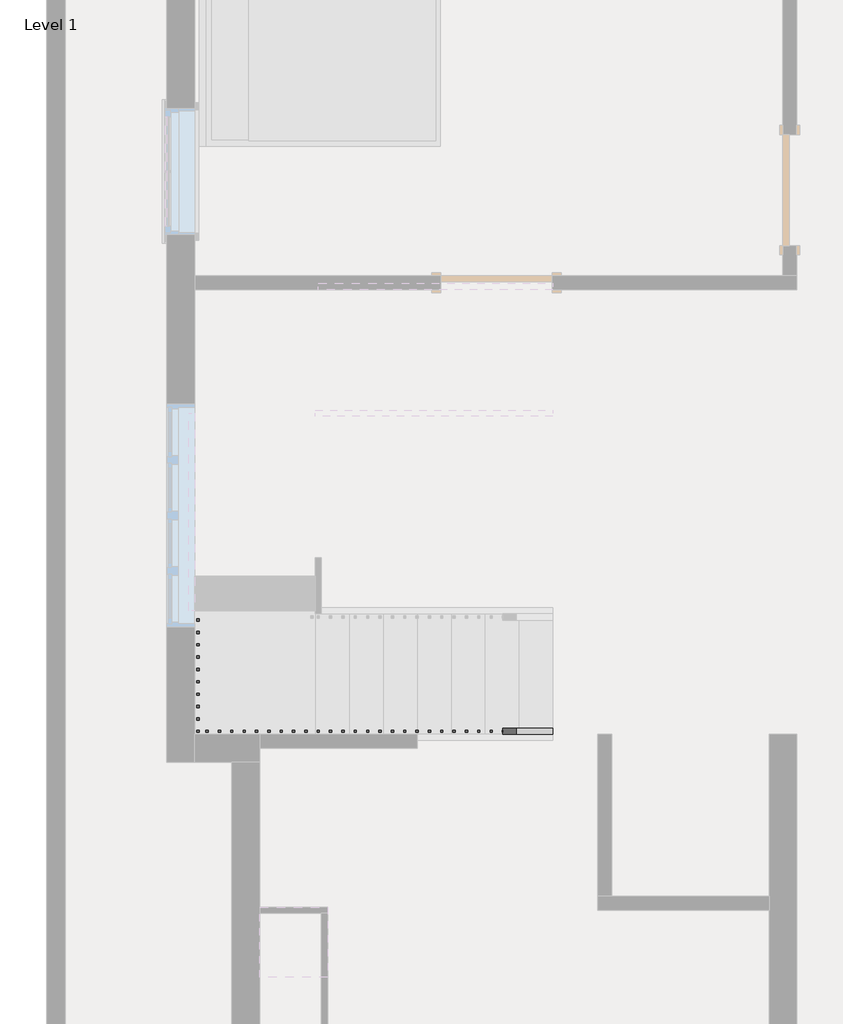
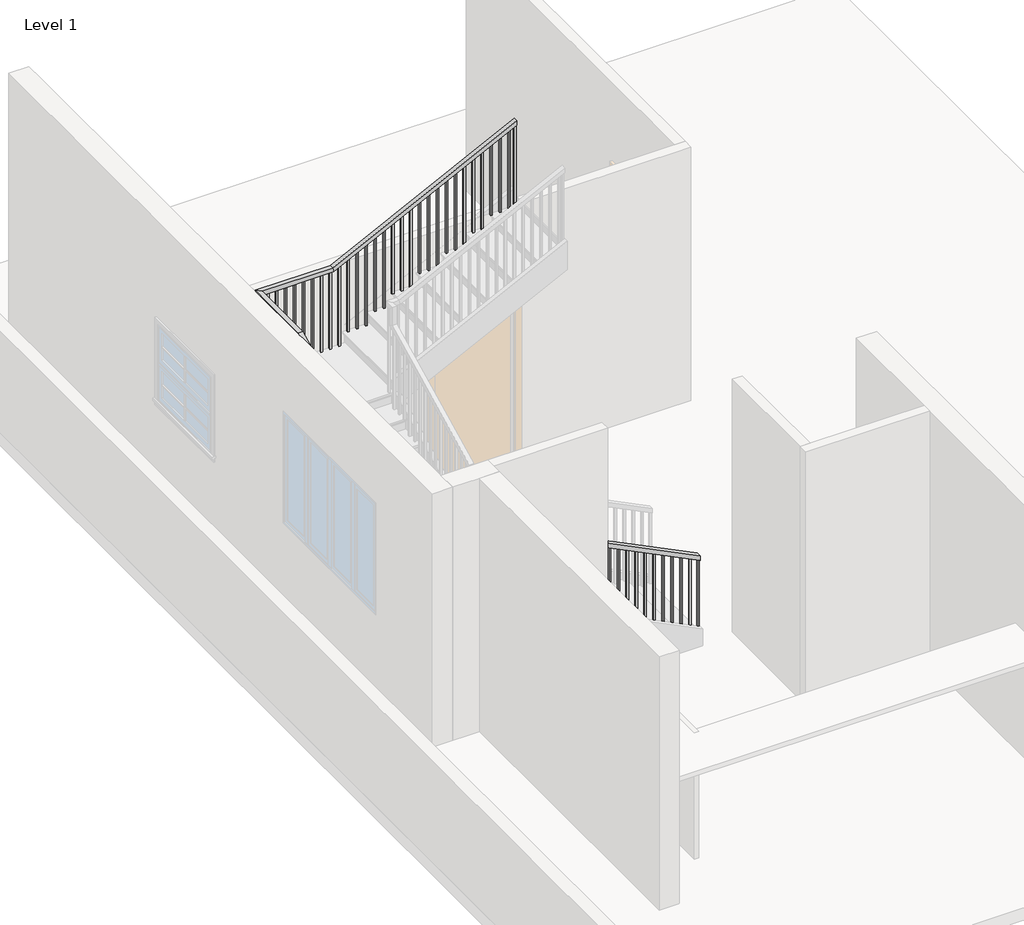
# One storey, part 3 of 8: 1 railing.
"""IFC4 building model written with IfcOpenShell, lengths in millimetres."""

from ifc_helpers import new_model, si_unit, frame, origin, place, context, project, spatial, polyline, outline, extrude, faceted_brep, element, save

model = new_model("IFC4")

# Units and contexts
model_context = context("Model", 3, world=origin())
ifc_project = project(units=[si_unit("LENGTHUNIT", "METRE", prefix="MILLI")], contexts=[model_context])

# Site, building, storey
site = spatial("IfcSite", under=ifc_project)
building = spatial("IfcBuilding", under=site)
storey = spatial("IfcBuildingStorey", under=building, Name="Level 1", Elevation=0.0)

# Railing
placement = place(None, origin())
element("IfcRailing", 1, ObjectType="Handrail - Rectangular", at=placement, inside=storey, context=model_context, shape_type="SolidModel", body=[
    faceted_brep([(-19769.8789184, -1118.4399287, 1052.9454545), (-19769.8789184, -1118.4399287, 996.242895), (-19769.8789184, -1067.6399287, 996.242895), (-19769.8789184, -1067.6399287, 1052.9454545), (-21865.3789184, -1118.4399287, 2092.0363636), (-21877.2824136, -1118.4399287, 2041.2363636), (-21877.2824136, -1067.6399287, 2041.2363636), (-21865.3789184, -1067.6399287, 2092.0363636), (-22716.2789184, -1118.4399287, 2041.2363636), (-22716.2789184, -1118.4399287, 2092.0363636), (-22716.2789184, -267.5399287, 2092.0363636), (-22716.2789184, -255.6364336, 2041.2363636), (-22665.4789184, -1067.6399287, 2041.2363636), (-22665.4789184, -255.6364336, 2041.2363636), (-22665.4789184, -1067.6399287, 2092.0363636), (-22665.4789184, -267.5399287, 2092.0363636), (-22716.2789184, 2539.1600713, 3011.0545455), (-22716.2789184, 2539.1600713, 3061.8545455), (-21865.3789184, 2539.1600713, 3061.8545455), (-21853.4754233, 2539.1600713, 3011.0545455), (-22665.4789184, 2488.3600713, 3011.0545455), (-21853.4754233, 2488.3600713, 3011.0545455), (-22665.4789184, 2488.3600713, 3061.8545455), (-21865.3789184, 2488.3600713, 3061.8545455), (-22716.2789184, 1688.2600713, 3061.8545455), (-22716.2789184, 1700.1635664, 3011.0545455), (-22665.4789184, 1700.1635664, 3011.0545455), (-22665.4789184, 1688.2600713, 3061.8545455), (-19769.8789184, 2539.1600713, 4100.9454545), (-19769.8789184, 2488.3600713, 4100.9454545), (-19769.8789184, 2488.3600713, 4044.242895), (-19769.8789184, 2539.1600713, 4044.242895)], [[[0, 1, 2, 3]], [[1, 0, 4, 5]], [[2, 1, 5, 6]], [[3, 2, 6, 7]], [[0, 3, 7, 4]], [[8, 9, 10, 11]], [[12, 8, 11, 13]], [[14, 12, 13, 15]], [[9, 14, 15, 10]], [[16, 17, 18, 19]], [[20, 16, 19, 21]], [[22, 20, 21, 23]], [[17, 22, 23, 18]], [[5, 4, 9, 8]], [[6, 5, 8, 12]], [[7, 6, 12, 14]], [[4, 7, 14, 9]], [[11, 10, 24, 25]], [[13, 11, 25, 26]], [[15, 13, 26, 27]], [[10, 15, 27, 24]], [[25, 24, 17, 16]], [[26, 25, 16, 20]], [[27, 26, 20, 22]], [[24, 27, 22, 17]], [[28, 29, 30, 31]], [[19, 18, 28, 31]], [[21, 19, 31, 30]], [[23, 21, 30, 29]], [[18, 23, 29, 28]]]),
    extrude(outline(polyline([(4001.7346305, -19855.6039184), (3048.0, -19855.6039184), (3048.0, -19836.5539184), (4011.1809115, -19836.5539184), (4001.7346305, -19855.6039184)])), frame((0.0, 2504.2350713, 0.0), z_axis=(0.0, 1.0, 0.0), x_axis=(0.0, 0.0, 1.0)), (0.0, 0.0, 1.0), 19.05),
    extrude(outline(polyline([(3951.3544652, -19957.2039184), (3048.0, -19957.2039184), (3048.0, -19938.1539184), (3960.8007462, -19938.1539184), (3951.3544652, -19957.2039184)])), frame((0.0, 2504.2350713, 0.0), z_axis=(0.0, 1.0, 0.0), x_axis=(0.0, 0.0, 1.0)), (0.0, 0.0, 1.0), 19.05),
    extrude(outline(polyline([(3900.9742999, -20058.8039184), (3048.0, -20058.8039184), (3048.0, -20039.7539184), (3910.4205809, -20039.7539184), (3900.9742999, -20058.8039184)])), frame((0.0, 2504.2350713, 0.0), z_axis=(0.0, 1.0, 0.0), x_axis=(0.0, 0.0, 1.0)), (0.0, 0.0, 1.0), 19.05),
    extrude(outline(polyline([(3850.5941346, -20160.4039184), (2909.4545455, -20160.4039184), (2909.4545455, -20141.3539184), (3860.0404156, -20141.3539184), (3850.5941346, -20160.4039184)])), frame((0.0, 2504.2350713, 0.0), z_axis=(0.0, 1.0, 0.0), x_axis=(0.0, 0.0, 1.0)), (0.0, 0.0, 1.0), 19.05),
    extrude(outline(polyline([(3800.2139693, -20262.0039184), (2909.4545455, -20262.0039184), (2909.4545455, -20242.9539184), (3809.6602503, -20242.9539184), (3800.2139693, -20262.0039184)])), frame((0.0, 2504.2350713, 0.0), z_axis=(0.0, 1.0, 0.0), x_axis=(0.0, 0.0, 1.0)), (0.0, 0.0, 1.0), 19.05),
    extrude(outline(polyline([(3749.833804, -20363.6039184), (2770.9090909, -20363.6039184), (2770.9090909, -20344.5539184), (3759.280085, -20344.5539184), (3749.833804, -20363.6039184)])), frame((0.0, 2504.2350713, 0.0), z_axis=(0.0, 1.0, 0.0), x_axis=(0.0, 0.0, 1.0)), (0.0, 0.0, 1.0), 19.05),
    extrude(outline(polyline([(3699.4536388, -20465.2039184), (2770.9090909, -20465.2039184), (2770.9090909, -20446.1539184), (3708.8999198, -20446.1539184), (3699.4536388, -20465.2039184)])), frame((0.0, 2504.2350713, 0.0), z_axis=(0.0, 1.0, 0.0), x_axis=(0.0, 0.0, 1.0)), (0.0, 0.0, 1.0), 19.05),
    extrude(outline(polyline([(3649.0734735, -20566.8039184), (2770.9090909, -20566.8039184), (2770.9090909, -20547.7539184), (3658.5197545, -20547.7539184), (3649.0734735, -20566.8039184)])), frame((0.0, 2504.2350713, 0.0), z_axis=(0.0, 1.0, 0.0), x_axis=(0.0, 0.0, 1.0)), (0.0, 0.0, 1.0), 19.05),
    extrude(outline(polyline([(3598.6933082, -20668.4039184), (2632.3636364, -20668.4039184), (2632.3636364, -20649.3539184), (3608.1395892, -20649.3539184), (3598.6933082, -20668.4039184)])), frame((0.0, 2504.2350713, 0.0), z_axis=(0.0, 1.0, 0.0), x_axis=(0.0, 0.0, 1.0)), (0.0, 0.0, 1.0), 19.05),
    extrude(outline(polyline([(3548.3131429, -20770.0039184), (2632.3636364, -20770.0039184), (2632.3636364, -20750.9539184), (3557.7594239, -20750.9539184), (3548.3131429, -20770.0039184)])), frame((0.0, 2504.2350713, 0.0), z_axis=(0.0, 1.0, 0.0), x_axis=(0.0, 0.0, 1.0)), (0.0, 0.0, 1.0), 19.05),
    extrude(outline(polyline([(3497.9329776, -20871.6039184), (2632.3636364, -20871.6039184), (2632.3636364, -20852.5539184), (3507.3792586, -20852.5539184), (3497.9329776, -20871.6039184)])), frame((0.0, 2504.2350713, 0.0), z_axis=(0.0, 1.0, 0.0), x_axis=(0.0, 0.0, 1.0)), (0.0, 0.0, 1.0), 19.05),
    extrude(outline(polyline([(3447.5528123, -20973.2039184), (2493.8181818, -20973.2039184), (2493.8181818, -20954.1539184), (3456.9990933, -20954.1539184), (3447.5528123, -20973.2039184)])), frame((0.0, 2504.2350713, 0.0), z_axis=(0.0, 1.0, 0.0), x_axis=(0.0, 0.0, 1.0)), (0.0, 0.0, 1.0), 19.05),
    extrude(outline(polyline([(3397.172647, -21074.8039184), (2493.8181818, -21074.8039184), (2493.8181818, -21055.7539184), (3406.618928, -21055.7539184), (3397.172647, -21074.8039184)])), frame((0.0, 2504.2350713, 0.0), z_axis=(0.0, 1.0, 0.0), x_axis=(0.0, 0.0, 1.0)), (0.0, 0.0, 1.0), 19.05),
    extrude(outline(polyline([(3346.7924817, -21176.4039184), (2493.8181818, -21176.4039184), (2493.8181818, -21157.3539184), (3356.2387627, -21157.3539184), (3346.7924817, -21176.4039184)])), frame((0.0, 2504.2350713, 0.0), z_axis=(0.0, 1.0, 0.0), x_axis=(0.0, 0.0, 1.0)), (0.0, 0.0, 1.0), 19.05),
    extrude(outline(polyline([(3296.4123164, -21278.0039184), (2355.2727273, -21278.0039184), (2355.2727273, -21258.9539184), (3305.8585974, -21258.9539184), (3296.4123164, -21278.0039184)])), frame((0.0, 2504.2350713, 0.0), z_axis=(0.0, 1.0, 0.0), x_axis=(0.0, 0.0, 1.0)), (0.0, 0.0, 1.0), 19.05),
    extrude(outline(polyline([(3246.0321512, -21379.6039184), (2355.2727273, -21379.6039184), (2355.2727273, -21360.5539184), (3255.4784321, -21360.5539184), (3246.0321512, -21379.6039184)])), frame((0.0, 2504.2350713, 0.0), z_axis=(0.0, 1.0, 0.0), x_axis=(0.0, 0.0, 1.0)), (0.0, 0.0, 1.0), 19.05),
    extrude(outline(polyline([(3195.6519859, -21481.2039184), (2216.7272727, -21481.2039184), (2216.7272727, -21462.1539184), (3205.0982669, -21462.1539184), (3195.6519859, -21481.2039184)])), frame((0.0, 2504.2350713, 0.0), z_axis=(0.0, 1.0, 0.0), x_axis=(0.0, 0.0, 1.0)), (0.0, 0.0, 1.0), 19.05),
    extrude(outline(polyline([(3145.2718206, -21582.8039184), (2216.7272727, -21582.8039184), (2216.7272727, -21563.7539184), (3154.7181016, -21563.7539184), (3145.2718206, -21582.8039184)])), frame((0.0, 2504.2350713, 0.0), z_axis=(0.0, 1.0, 0.0), x_axis=(0.0, 0.0, 1.0)), (0.0, 0.0, 1.0), 19.05),
    extrude(outline(polyline([(3094.8916553, -21684.4039184), (2216.7272727, -21684.4039184), (2216.7272727, -21665.3539184), (3104.3379363, -21665.3539184), (3094.8916553, -21684.4039184)])), frame((0.0, 2504.2350713, 0.0), z_axis=(0.0, 1.0, 0.0), x_axis=(0.0, 0.0, 1.0)), (0.0, 0.0, 1.0), 19.05),
    extrude(outline(polyline([(3044.51149, -21786.0039184), (2078.1818182, -21786.0039184), (2078.1818182, -21766.9539184), (3053.957771, -21766.9539184), (3044.51149, -21786.0039184)])), frame((0.0, 2504.2350713, 0.0), z_axis=(0.0, 1.0, 0.0), x_axis=(0.0, 0.0, 1.0)), (0.0, 0.0, 1.0), 19.05),
    extrude(outline(polyline([(-21887.6039184, 2523.2850713), (-21868.5539184, 2523.2850713), (-21868.5539184, 2504.2350713), (-21887.6039184, 2504.2350713), (-21887.6039184, 2523.2850713)])), frame((0.0, 0.0, 2078.1818182), z_axis=(0.0, 0.0, 1.0), x_axis=(1.0, 0.0, 0.0)), (0.0, 0.0, 1.0), 932.8727273),
    extrude(outline(polyline([(-21989.2039184, 2523.2850713), (-21970.1539184, 2523.2850713), (-21970.1539184, 2504.2350713), (-21989.2039184, 2504.2350713), (-21989.2039184, 2523.2850713)])), frame((0.0, 0.0, 2078.1818182), z_axis=(0.0, 0.0, 1.0), x_axis=(1.0, 0.0, 0.0)), (0.0, 0.0, 1.0), 932.8727273),
    extrude(outline(polyline([(-22090.8039184, 2523.2850713), (-22071.7539184, 2523.2850713), (-22071.7539184, 2504.2350713), (-22090.8039184, 2504.2350713), (-22090.8039184, 2523.2850713)])), frame((0.0, 0.0, 2078.1818182), z_axis=(0.0, 0.0, 1.0), x_axis=(1.0, 0.0, 0.0)), (0.0, 0.0, 1.0), 932.8727273),
    extrude(outline(polyline([(-22192.4039184, 2523.2850713), (-22173.3539184, 2523.2850713), (-22173.3539184, 2504.2350713), (-22192.4039184, 2504.2350713), (-22192.4039184, 2523.2850713)])), frame((0.0, 0.0, 2078.1818182), z_axis=(0.0, 0.0, 1.0), x_axis=(1.0, 0.0, 0.0)), (0.0, 0.0, 1.0), 932.8727273),
    extrude(outline(polyline([(-22294.0039184, 2523.2850713), (-22274.9539184, 2523.2850713), (-22274.9539184, 2504.2350713), (-22294.0039184, 2504.2350713), (-22294.0039184, 2523.2850713)])), frame((0.0, 0.0, 2078.1818182), z_axis=(0.0, 0.0, 1.0), x_axis=(1.0, 0.0, 0.0)), (0.0, 0.0, 1.0), 932.8727273),
    extrude(outline(polyline([(-22395.6039184, 2523.2850713), (-22376.5539184, 2523.2850713), (-22376.5539184, 2504.2350713), (-22395.6039184, 2504.2350713), (-22395.6039184, 2523.2850713)])), frame((0.0, 0.0, 2078.1818182), z_axis=(0.0, 0.0, 1.0), x_axis=(1.0, 0.0, 0.0)), (0.0, 0.0, 1.0), 932.8727273),
    extrude(outline(polyline([(-22497.2039184, 2523.2850713), (-22478.1539184, 2523.2850713), (-22478.1539184, 2504.2350713), (-22497.2039184, 2504.2350713), (-22497.2039184, 2523.2850713)])), frame((0.0, 0.0, 2078.1818182), z_axis=(0.0, 0.0, 1.0), x_axis=(1.0, 0.0, 0.0)), (0.0, 0.0, 1.0), 932.8727273),
    extrude(outline(polyline([(-22598.8039184, 2523.2850713), (-22579.7539184, 2523.2850713), (-22579.7539184, 2504.2350713), (-22598.8039184, 2504.2350713), (-22598.8039184, 2523.2850713)])), frame((0.0, 0.0, 2078.1818182), z_axis=(0.0, 0.0, 1.0), x_axis=(1.0, 0.0, 0.0)), (0.0, 0.0, 1.0), 932.8727273),
    extrude(outline(polyline([(-22700.4039184, 2453.4350713), (-22700.4039184, 2472.4850713), (-22681.3539184, 2472.4850713), (-22681.3539184, 2453.4350713), (-22700.4039184, 2453.4350713)])), frame((0.0, 0.0, 2078.1818182), z_axis=(0.0, 0.0, 1.0), x_axis=(1.0, 0.0, 0.0)), (0.0, 0.0, 1.0), 932.8727273),
    extrude(outline(polyline([(-22700.4039184, 2351.8350713), (-22700.4039184, 2370.8850713), (-22681.3539184, 2370.8850713), (-22681.3539184, 2351.8350713), (-22700.4039184, 2351.8350713)])), frame((0.0, 0.0, 2078.1818182), z_axis=(0.0, 0.0, 1.0), x_axis=(1.0, 0.0, 0.0)), (0.0, 0.0, 1.0), 932.8727273),
    extrude(outline(polyline([(-22700.4039184, 2250.2350713), (-22700.4039184, 2269.2850713), (-22681.3539184, 2269.2850713), (-22681.3539184, 2250.2350713), (-22700.4039184, 2250.2350713)])), frame((0.0, 0.0, 2078.1818182), z_axis=(0.0, 0.0, 1.0), x_axis=(1.0, 0.0, 0.0)), (0.0, 0.0, 1.0), 932.8727273),
    extrude(outline(polyline([(-22700.4039184, 2148.6350713), (-22700.4039184, 2167.6850713), (-22681.3539184, 2167.6850713), (-22681.3539184, 2148.6350713), (-22700.4039184, 2148.6350713)])), frame((0.0, 0.0, 2078.1818182), z_axis=(0.0, 0.0, 1.0), x_axis=(1.0, 0.0, 0.0)), (0.0, 0.0, 1.0), 932.8727273),
    extrude(outline(polyline([(-22700.4039184, 2047.0350713), (-22700.4039184, 2066.0850713), (-22681.3539184, 2066.0850713), (-22681.3539184, 2047.0350713), (-22700.4039184, 2047.0350713)])), frame((0.0, 0.0, 2078.1818182), z_axis=(0.0, 0.0, 1.0), x_axis=(1.0, 0.0, 0.0)), (0.0, 0.0, 1.0), 932.8727273),
    extrude(outline(polyline([(-22700.4039184, 1945.4350713), (-22700.4039184, 1964.4850713), (-22681.3539184, 1964.4850713), (-22681.3539184, 1945.4350713), (-22700.4039184, 1945.4350713)])), frame((0.0, 0.0, 2078.1818182), z_axis=(0.0, 0.0, 1.0), x_axis=(1.0, 0.0, 0.0)), (0.0, 0.0, 1.0), 932.8727273),
    extrude(outline(polyline([(-22700.4039184, 1843.8350713), (-22700.4039184, 1862.8850713), (-22681.3539184, 1862.8850713), (-22681.3539184, 1843.8350713), (-22700.4039184, 1843.8350713)])), frame((0.0, 0.0, 2078.1818182), z_axis=(0.0, 0.0, 1.0), x_axis=(1.0, 0.0, 0.0)), (0.0, 0.0, 1.0), 932.8727273),
    extrude(outline(polyline([(-22700.4039184, 1742.2350713), (-22700.4039184, 1761.2850713), (-22681.3539184, 1761.2850713), (-22681.3539184, 1742.2350713), (-22700.4039184, 1742.2350713)])), frame((0.0, 0.0, 2078.1818182), z_axis=(0.0, 0.0, 1.0), x_axis=(1.0, 0.0, 0.0)), (0.0, 0.0, 1.0), 932.8727273),
    extrude(outline(polyline([(1659.6850713, 2990.9825644), (1659.6850713, 2078.1818182), (1640.6350713, 2078.1818182), (1640.6350713, 2981.5362834), (1659.6850713, 2990.9825644)])), frame((-22700.4039184, 0.0, 0.0), z_axis=(1.0, 0.0, 0.0), x_axis=(0.0, 1.0, 0.0)), (0.0, 0.0, 1.0), 19.05),
    extrude(outline(polyline([(1558.0850713, 2940.6023991), (1558.0850713, 2078.1818182), (1539.0350713, 2078.1818182), (1539.0350713, 2931.1561181), (1558.0850713, 2940.6023991)])), frame((-22700.4039184, 0.0, 0.0), z_axis=(1.0, 0.0, 0.0), x_axis=(0.0, 1.0, 0.0)), (0.0, 0.0, 1.0), 19.05),
    extrude(outline(polyline([(1456.4850713, 2890.2222338), (1456.4850713, 1939.6363636), (1437.4350713, 1939.6363636), (1437.4350713, 2880.7759528), (1456.4850713, 2890.2222338)])), frame((-22700.4039184, 0.0, 0.0), z_axis=(1.0, 0.0, 0.0), x_axis=(0.0, 1.0, 0.0)), (0.0, 0.0, 1.0), 19.05),
    extrude(outline(polyline([(1354.8850713, 2839.8420685), (1354.8850713, 1939.6363636), (1335.8350713, 1939.6363636), (1335.8350713, 2830.3957875), (1354.8850713, 2839.8420685)])), frame((-22700.4039184, 0.0, 0.0), z_axis=(1.0, 0.0, 0.0), x_axis=(0.0, 1.0, 0.0)), (0.0, 0.0, 1.0), 19.05),
    extrude(outline(polyline([(1253.2850713, 2789.4619032), (1253.2850713, 1801.0909091), (1234.2350713, 1801.0909091), (1234.2350713, 2780.0156222), (1253.2850713, 2789.4619032)])), frame((-22700.4039184, 0.0, 0.0), z_axis=(1.0, 0.0, 0.0), x_axis=(0.0, 1.0, 0.0)), (0.0, 0.0, 1.0), 19.05),
    extrude(outline(polyline([(1151.6850713, 2739.0817379), (1151.6850713, 1801.0909091), (1132.6350713, 1801.0909091), (1132.6350713, 2729.6354569), (1151.6850713, 2739.0817379)])), frame((-22700.4039184, 0.0, 0.0), z_axis=(1.0, 0.0, 0.0), x_axis=(0.0, 1.0, 0.0)), (0.0, 0.0, 1.0), 19.05),
    extrude(outline(polyline([(1050.0850713, 2688.7015726), (1050.0850713, 1801.0909091), (1031.0350713, 1801.0909091), (1031.0350713, 2679.2552917), (1050.0850713, 2688.7015726)])), frame((-22700.4039184, 0.0, 0.0), z_axis=(1.0, 0.0, 0.0), x_axis=(0.0, 1.0, 0.0)), (0.0, 0.0, 1.0), 19.05),
    extrude(outline(polyline([(948.4850713, 2638.3214074), (948.4850713, 1662.5454545), (929.4350713, 1662.5454545), (929.4350713, 2628.8751264), (948.4850713, 2638.3214074)])), frame((-22700.4039184, 0.0, 0.0), z_axis=(1.0, 0.0, 0.0), x_axis=(0.0, 1.0, 0.0)), (0.0, 0.0, 1.0), 19.05),
    extrude(outline(polyline([(846.8850713, 2587.9412421), (846.8850713, 1662.5454545), (827.8350713, 1662.5454545), (827.8350713, 2578.4949611), (846.8850713, 2587.9412421)])), frame((-22700.4039184, 0.0, 0.0), z_axis=(1.0, 0.0, 0.0), x_axis=(0.0, 1.0, 0.0)), (0.0, 0.0, 1.0), 19.05),
    extrude(outline(polyline([(745.2850713, 2537.5610768), (745.2850713, 1662.5454545), (726.2350713, 1662.5454545), (726.2350713, 2528.1147958), (745.2850713, 2537.5610768)])), frame((-22700.4039184, 0.0, 0.0), z_axis=(1.0, 0.0, 0.0), x_axis=(0.0, 1.0, 0.0)), (0.0, 0.0, 1.0), 19.05),
    extrude(outline(polyline([(643.6850713, 2487.1809115), (643.6850713, 1524.0), (624.6350713, 1524.0), (624.6350713, 2477.7346305), (643.6850713, 2487.1809115)])), frame((-22700.4039184, 0.0, 0.0), z_axis=(1.0, 0.0, 0.0), x_axis=(0.0, 1.0, 0.0)), (0.0, 0.0, 1.0), 19.05),
    extrude(outline(polyline([(542.0850713, 2436.8007462), (542.0850713, 1524.0), (523.0350713, 1524.0), (523.0350713, 2427.3544652), (542.0850713, 2436.8007462)])), frame((-22700.4039184, 0.0, 0.0), z_axis=(1.0, 0.0, 0.0), x_axis=(0.0, 1.0, 0.0)), (0.0, 0.0, 1.0), 19.05),
    extrude(outline(polyline([(440.4850713, 2386.4205809), (440.4850713, 1524.0), (421.4350713, 1524.0), (421.4350713, 2376.9742999), (440.4850713, 2386.4205809)])), frame((-22700.4039184, 0.0, 0.0), z_axis=(1.0, 0.0, 0.0), x_axis=(0.0, 1.0, 0.0)), (0.0, 0.0, 1.0), 19.05),
    extrude(outline(polyline([(338.8850713, 2336.0404156), (338.8850713, 1385.4545455), (319.8350713, 1385.4545455), (319.8350713, 2326.5941346), (338.8850713, 2336.0404156)])), frame((-22700.4039184, 0.0, 0.0), z_axis=(1.0, 0.0, 0.0), x_axis=(0.0, 1.0, 0.0)), (0.0, 0.0, 1.0), 19.05),
    extrude(outline(polyline([(237.2850713, 2285.6602503), (237.2850713, 1385.4545455), (218.2350713, 1385.4545455), (218.2350713, 2276.2139693), (237.2850713, 2285.6602503)])), frame((-22700.4039184, 0.0, 0.0), z_axis=(1.0, 0.0, 0.0), x_axis=(0.0, 1.0, 0.0)), (0.0, 0.0, 1.0), 19.05),
    extrude(outline(polyline([(135.6850713, 2235.280085), (135.6850713, 1246.9090909), (116.6350713, 1246.9090909), (116.6350713, 2225.833804), (135.6850713, 2235.280085)])), frame((-22700.4039184, 0.0, 0.0), z_axis=(1.0, 0.0, 0.0), x_axis=(0.0, 1.0, 0.0)), (0.0, 0.0, 1.0), 19.05),
    extrude(outline(polyline([(34.0850713, 2184.8999198), (34.0850713, 1246.9090909), (15.0350713, 1246.9090909), (15.0350713, 2175.4536388), (34.0850713, 2184.8999198)])), frame((-22700.4039184, 0.0, 0.0), z_axis=(1.0, 0.0, 0.0), x_axis=(0.0, 1.0, 0.0)), (0.0, 0.0, 1.0), 19.05),
    extrude(outline(polyline([(-67.5149287, 2134.5197545), (-67.5149287, 1246.9090909), (-86.5649287, 1246.9090909), (-86.5649287, 2125.0734735), (-67.5149287, 2134.5197545)])), frame((-22700.4039184, 0.0, 0.0), z_axis=(1.0, 0.0, 0.0), x_axis=(0.0, 1.0, 0.0)), (0.0, 0.0, 1.0), 19.05),
    extrude(outline(polyline([(-169.1149287, 2084.1395892), (-169.1149287, 1108.3636364), (-188.1649287, 1108.3636364), (-188.1649287, 2074.6933082), (-169.1149287, 2084.1395892)])), frame((-22700.4039184, 0.0, 0.0), z_axis=(1.0, 0.0, 0.0), x_axis=(0.0, 1.0, 0.0)), (0.0, 0.0, 1.0), 19.05),
    extrude(outline(polyline([(-22700.4039184, -289.7649287), (-22700.4039184, -270.7149287), (-22681.3539184, -270.7149287), (-22681.3539184, -289.7649287), (-22700.4039184, -289.7649287)])), frame((0.0, 0.0, 1108.3636364), z_axis=(0.0, 0.0, 1.0), x_axis=(1.0, 0.0, 0.0)), (0.0, 0.0, 1.0), 932.8727273),
    extrude(outline(polyline([(-22700.4039184, -391.3649287), (-22700.4039184, -372.3149287), (-22681.3539184, -372.3149287), (-22681.3539184, -391.3649287), (-22700.4039184, -391.3649287)])), frame((0.0, 0.0, 1108.3636364), z_axis=(0.0, 0.0, 1.0), x_axis=(1.0, 0.0, 0.0)), (0.0, 0.0, 1.0), 932.8727273),
    extrude(outline(polyline([(-22700.4039184, -492.9649287), (-22700.4039184, -473.9149287), (-22681.3539184, -473.9149287), (-22681.3539184, -492.9649287), (-22700.4039184, -492.9649287)])), frame((0.0, 0.0, 1108.3636364), z_axis=(0.0, 0.0, 1.0), x_axis=(1.0, 0.0, 0.0)), (0.0, 0.0, 1.0), 932.8727273),
    extrude(outline(polyline([(-22700.4039184, -594.5649287), (-22700.4039184, -575.5149287), (-22681.3539184, -575.5149287), (-22681.3539184, -594.5649287), (-22700.4039184, -594.5649287)])), frame((0.0, 0.0, 1108.3636364), z_axis=(0.0, 0.0, 1.0), x_axis=(1.0, 0.0, 0.0)), (0.0, 0.0, 1.0), 932.8727273),
    extrude(outline(polyline([(-22700.4039184, -696.1649287), (-22700.4039184, -677.1149287), (-22681.3539184, -677.1149287), (-22681.3539184, -696.1649287), (-22700.4039184, -696.1649287)])), frame((0.0, 0.0, 1108.3636364), z_axis=(0.0, 0.0, 1.0), x_axis=(1.0, 0.0, 0.0)), (0.0, 0.0, 1.0), 932.8727273),
    extrude(outline(polyline([(-22700.4039184, -797.7649287), (-22700.4039184, -778.7149287), (-22681.3539184, -778.7149287), (-22681.3539184, -797.7649287), (-22700.4039184, -797.7649287)])), frame((0.0, 0.0, 1108.3636364), z_axis=(0.0, 0.0, 1.0), x_axis=(1.0, 0.0, 0.0)), (0.0, 0.0, 1.0), 932.8727273),
    extrude(outline(polyline([(-22700.4039184, -899.3649287), (-22700.4039184, -880.3149287), (-22681.3539184, -880.3149287), (-22681.3539184, -899.3649287), (-22700.4039184, -899.3649287)])), frame((0.0, 0.0, 1108.3636364), z_axis=(0.0, 0.0, 1.0), x_axis=(1.0, 0.0, 0.0)), (0.0, 0.0, 1.0), 932.8727273),
    extrude(outline(polyline([(-22700.4039184, -1000.9649287), (-22700.4039184, -981.9149287), (-22681.3539184, -981.9149287), (-22681.3539184, -1000.9649287), (-22700.4039184, -1000.9649287)])), frame((0.0, 0.0, 1108.3636364), z_axis=(0.0, 0.0, 1.0), x_axis=(1.0, 0.0, 0.0)), (0.0, 0.0, 1.0), 932.8727273),
    extrude(outline(polyline([(-22605.1539184, -1102.5649287), (-22624.2039184, -1102.5649287), (-22624.2039184, -1083.5149287), (-22605.1539184, -1083.5149287), (-22605.1539184, -1102.5649287)])), frame((0.0, 0.0, 1108.3636364), z_axis=(0.0, 0.0, 1.0), x_axis=(1.0, 0.0, 0.0)), (0.0, 0.0, 1.0), 932.8727273),
    extrude(outline(polyline([(-22503.5539184, -1102.5649287), (-22522.6039184, -1102.5649287), (-22522.6039184, -1083.5149287), (-22503.5539184, -1083.5149287), (-22503.5539184, -1102.5649287)])), frame((0.0, 0.0, 1108.3636364), z_axis=(0.0, 0.0, 1.0), x_axis=(1.0, 0.0, 0.0)), (0.0, 0.0, 1.0), 932.8727273),
    extrude(outline(polyline([(-22401.9539184, -1102.5649287), (-22421.0039184, -1102.5649287), (-22421.0039184, -1083.5149287), (-22401.9539184, -1083.5149287), (-22401.9539184, -1102.5649287)])), frame((0.0, 0.0, 1108.3636364), z_axis=(0.0, 0.0, 1.0), x_axis=(1.0, 0.0, 0.0)), (0.0, 0.0, 1.0), 932.8727273),
    extrude(outline(polyline([(-22300.3539184, -1102.5649287), (-22319.4039184, -1102.5649287), (-22319.4039184, -1083.5149287), (-22300.3539184, -1083.5149287), (-22300.3539184, -1102.5649287)])), frame((0.0, 0.0, 1108.3636364), z_axis=(0.0, 0.0, 1.0), x_axis=(1.0, 0.0, 0.0)), (0.0, 0.0, 1.0), 932.8727273),
    extrude(outline(polyline([(-22198.7539184, -1102.5649287), (-22217.8039184, -1102.5649287), (-22217.8039184, -1083.5149287), (-22198.7539184, -1083.5149287), (-22198.7539184, -1102.5649287)])), frame((0.0, 0.0, 1108.3636364), z_axis=(0.0, 0.0, 1.0), x_axis=(1.0, 0.0, 0.0)), (0.0, 0.0, 1.0), 932.8727273),
    extrude(outline(polyline([(-22097.1539184, -1102.5649287), (-22116.2039184, -1102.5649287), (-22116.2039184, -1083.5149287), (-22097.1539184, -1083.5149287), (-22097.1539184, -1102.5649287)])), frame((0.0, 0.0, 1108.3636364), z_axis=(0.0, 0.0, 1.0), x_axis=(1.0, 0.0, 0.0)), (0.0, 0.0, 1.0), 932.8727273),
    extrude(outline(polyline([(-21995.5539184, -1102.5649287), (-22014.6039184, -1102.5649287), (-22014.6039184, -1083.5149287), (-21995.5539184, -1083.5149287), (-21995.5539184, -1102.5649287)])), frame((0.0, 0.0, 1108.3636364), z_axis=(0.0, 0.0, 1.0), x_axis=(1.0, 0.0, 0.0)), (0.0, 0.0, 1.0), 932.8727273),
    extrude(outline(polyline([(-21893.9539184, -1102.5649287), (-21913.0039184, -1102.5649287), (-21913.0039184, -1083.5149287), (-21893.9539184, -1083.5149287), (-21893.9539184, -1102.5649287)])), frame((0.0, 0.0, 1108.3636364), z_axis=(0.0, 0.0, 1.0), x_axis=(1.0, 0.0, 0.0)), (0.0, 0.0, 1.0), 932.8727273),
    extrude(outline(polyline([(2008.5693412, -21811.4039184), (1108.3636364, -21811.4039184), (1108.3636364, -21792.3539184), (1999.1230602, -21792.3539184), (2008.5693412, -21811.4039184)])), frame((0.0, -1102.5649287, 0.0), z_axis=(0.0, 1.0, 0.0), x_axis=(0.0, 0.0, 1.0)), (0.0, 0.0, 1.0), 19.05),
    extrude(outline(polyline([(1958.189176, -21709.8039184), (969.8181818, -21709.8039184), (969.8181818, -21690.7539184), (1948.742895, -21690.7539184), (1958.189176, -21709.8039184)])), frame((0.0, -1102.5649287, 0.0), z_axis=(0.0, 1.0, 0.0), x_axis=(0.0, 0.0, 1.0)), (0.0, 0.0, 1.0), 19.05),
    extrude(outline(polyline([(1907.8090107, -21608.2039184), (969.8181818, -21608.2039184), (969.8181818, -21589.1539184), (1898.3627297, -21589.1539184), (1907.8090107, -21608.2039184)])), frame((0.0, -1102.5649287, 0.0), z_axis=(0.0, 1.0, 0.0), x_axis=(0.0, 0.0, 1.0)), (0.0, 0.0, 1.0), 19.05),
    extrude(outline(polyline([(1857.4288454, -21506.6039184), (969.8181818, -21506.6039184), (969.8181818, -21487.5539184), (1847.9825644, -21487.5539184), (1857.4288454, -21506.6039184)])), frame((0.0, -1102.5649287, 0.0), z_axis=(0.0, 1.0, 0.0), x_axis=(0.0, 0.0, 1.0)), (0.0, 0.0, 1.0), 19.05),
    extrude(outline(polyline([(1807.0486801, -21405.0039184), (831.2727273, -21405.0039184), (831.2727273, -21385.9539184), (1797.6023991, -21385.9539184), (1807.0486801, -21405.0039184)])), frame((0.0, -1102.5649287, 0.0), z_axis=(0.0, 1.0, 0.0), x_axis=(0.0, 0.0, 1.0)), (0.0, 0.0, 1.0), 19.05),
    extrude(outline(polyline([(1756.6685148, -21303.4039184), (831.2727273, -21303.4039184), (831.2727273, -21284.3539184), (1747.2222338, -21284.3539184), (1756.6685148, -21303.4039184)])), frame((0.0, -1102.5649287, 0.0), z_axis=(0.0, 1.0, 0.0), x_axis=(0.0, 0.0, 1.0)), (0.0, 0.0, 1.0), 19.05),
    extrude(outline(polyline([(1706.2883495, -21201.8039184), (831.2727273, -21201.8039184), (831.2727273, -21182.7539184), (1696.8420685, -21182.7539184), (1706.2883495, -21201.8039184)])), frame((0.0, -1102.5649287, 0.0), z_axis=(0.0, 1.0, 0.0), x_axis=(0.0, 0.0, 1.0)), (0.0, 0.0, 1.0), 19.05),
    extrude(outline(polyline([(1655.9081842, -21100.2039184), (692.7272727, -21100.2039184), (692.7272727, -21081.1539184), (1646.4619032, -21081.1539184), (1655.9081842, -21100.2039184)])), frame((0.0, -1102.5649287, 0.0), z_axis=(0.0, 1.0, 0.0), x_axis=(0.0, 0.0, 1.0)), (0.0, 0.0, 1.0), 19.05),
    extrude(outline(polyline([(1605.5280189, -20998.6039184), (692.7272727, -20998.6039184), (692.7272727, -20979.5539184), (1596.0817379, -20979.5539184), (1605.5280189, -20998.6039184)])), frame((0.0, -1102.5649287, 0.0), z_axis=(0.0, 1.0, 0.0), x_axis=(0.0, 0.0, 1.0)), (0.0, 0.0, 1.0), 19.05),
    extrude(outline(polyline([(1555.1478536, -20897.0039184), (692.7272727, -20897.0039184), (692.7272727, -20877.9539184), (1545.7015726, -20877.9539184), (1555.1478536, -20897.0039184)])), frame((0.0, -1102.5649287, 0.0), z_axis=(0.0, 1.0, 0.0), x_axis=(0.0, 0.0, 1.0)), (0.0, 0.0, 1.0), 19.05),
    extrude(outline(polyline([(1504.7676883, -20795.4039184), (554.1818182, -20795.4039184), (554.1818182, -20776.3539184), (1495.3214074, -20776.3539184), (1504.7676883, -20795.4039184)])), frame((0.0, -1102.5649287, 0.0), z_axis=(0.0, 1.0, 0.0), x_axis=(0.0, 0.0, 1.0)), (0.0, 0.0, 1.0), 19.05),
    extrude(outline(polyline([(1454.3875231, -20693.8039184), (554.1818182, -20693.8039184), (554.1818182, -20674.7539184), (1444.9412421, -20674.7539184), (1454.3875231, -20693.8039184)])), frame((0.0, -1102.5649287, 0.0), z_axis=(0.0, 1.0, 0.0), x_axis=(0.0, 0.0, 1.0)), (0.0, 0.0, 1.0), 19.05),
    extrude(outline(polyline([(1404.0073578, -20592.2039184), (415.6363636, -20592.2039184), (415.6363636, -20573.1539184), (1394.5610768, -20573.1539184), (1404.0073578, -20592.2039184)])), frame((0.0, -1102.5649287, 0.0), z_axis=(0.0, 1.0, 0.0), x_axis=(0.0, 0.0, 1.0)), (0.0, 0.0, 1.0), 19.05),
    extrude(outline(polyline([(1353.6271925, -20490.6039184), (415.6363636, -20490.6039184), (415.6363636, -20471.5539184), (1344.1809115, -20471.5539184), (1353.6271925, -20490.6039184)])), frame((0.0, -1102.5649287, 0.0), z_axis=(0.0, 1.0, 0.0), x_axis=(0.0, 0.0, 1.0)), (0.0, 0.0, 1.0), 19.05),
    extrude(outline(polyline([(1303.2470272, -20389.0039184), (415.6363636, -20389.0039184), (415.6363636, -20369.9539184), (1293.8007462, -20369.9539184), (1303.2470272, -20389.0039184)])), frame((0.0, -1102.5649287, 0.0), z_axis=(0.0, 1.0, 0.0), x_axis=(0.0, 0.0, 1.0)), (0.0, 0.0, 1.0), 19.05),
    extrude(outline(polyline([(1252.8668619, -20287.4039184), (277.0909091, -20287.4039184), (277.0909091, -20268.3539184), (1243.4205809, -20268.3539184), (1252.8668619, -20287.4039184)])), frame((0.0, -1102.5649287, 0.0), z_axis=(0.0, 1.0, 0.0), x_axis=(0.0, 0.0, 1.0)), (0.0, 0.0, 1.0), 19.05),
    extrude(outline(polyline([(1202.4866966, -20185.8039184), (277.0909091, -20185.8039184), (277.0909091, -20166.7539184), (1193.0404156, -20166.7539184), (1202.4866966, -20185.8039184)])), frame((0.0, -1102.5649287, 0.0), z_axis=(0.0, 1.0, 0.0), x_axis=(0.0, 0.0, 1.0)), (0.0, 0.0, 1.0), 19.05),
    extrude(outline(polyline([(1152.1065313, -20084.2039184), (277.0909091, -20084.2039184), (277.0909091, -20065.1539184), (1142.6602503, -20065.1539184), (1152.1065313, -20084.2039184)])), frame((0.0, -1102.5649287, 0.0), z_axis=(0.0, 1.0, 0.0), x_axis=(0.0, 0.0, 1.0)), (0.0, 0.0, 1.0), 19.05),
    extrude(outline(polyline([(1101.726366, -19982.6039184), (138.5454545, -19982.6039184), (138.5454545, -19963.5539184), (1092.280085, -19963.5539184), (1101.726366, -19982.6039184)])), frame((0.0, -1102.5649287, 0.0), z_axis=(0.0, 1.0, 0.0), x_axis=(0.0, 0.0, 1.0)), (0.0, 0.0, 1.0), 19.05),
    extrude(outline(polyline([(1051.3462007, -19881.0039184), (138.5454545, -19881.0039184), (138.5454545, -19861.9539184), (1041.8999198, -19861.9539184), (1051.3462007, -19881.0039184)])), frame((0.0, -1102.5649287, 0.0), z_axis=(0.0, 1.0, 0.0), x_axis=(0.0, 0.0, 1.0)), (0.0, 0.0, 1.0), 19.05),
    extrude(outline(polyline([(-22700.4039184, 2504.2350713), (-22700.4039184, 2523.2850713), (-22681.3539184, 2523.2850713), (-22681.3539184, 2504.2350713), (-22700.4039184, 2504.2350713)])), frame((0.0, 0.0, 2078.1818182), z_axis=(0.0, 0.0, 1.0), x_axis=(1.0, 0.0, 0.0)), (0.0, 0.0, 1.0), 932.8727273),
    extrude(outline(polyline([(-22681.3539184, -1102.5649287), (-22700.4039184, -1102.5649287), (-22700.4039184, -1083.5149287), (-22681.3539184, -1083.5149287), (-22681.3539184, -1102.5649287)])), frame((0.0, 0.0, 1108.3636364), z_axis=(0.0, 0.0, 1.0), x_axis=(1.0, 0.0, 0.0)), (0.0, 0.0, 1.0), 932.8727273),
    extrude(outline(polyline([(4034.796614, -19788.9289184), (3048.0, -19788.9289184), (3048.0, -19769.8789184), (4044.242895, -19769.8789184), (4034.796614, -19788.9289184)])), frame((0.0, 2504.2350713, 0.0), z_axis=(0.0, 1.0, 0.0), x_axis=(0.0, 0.0, 1.0)), (0.0, 0.0, 1.0), 19.05),
    extrude(outline(polyline([(1005.689176, -19788.9289184), (138.5454545, -19788.9289184), (138.5454545, -19769.8789184), (996.242895, -19769.8789184), (1005.689176, -19788.9289184)])), frame((0.0, -1102.5649287, 0.0), z_axis=(0.0, 1.0, 0.0), x_axis=(0.0, 0.0, 1.0)), (0.0, 0.0, 1.0), 19.05),
])

save(model, "model.ifc")

# Revit data of these elements
# Type "Handrail - Rectangular"
#   Assembly Code = "C2010400"
#   built-in parameter 1008612 = 0.0416667 (stored number, unit not read)
#   built-in parameter 1008611 = 0.0416667 (stored number, unit not read)
#   built-in parameter 1008609 = 0.333333 (stored number, unit not read)
#   built-in parameter 1008604 = 0.166667 (stored number, unit not read)
#   built-in parameter 1008603 = 0.166667 (stored number, unit not read)
#   Railing Height = 3' - 0"
#   built-in parameter 1008630 = 2
#   built-in parameter 1008610 = 2
#   built-in parameter 1008618 = Baluster - Square : 3/4"
# Element 1 (IfcRailing, "Handrail - Rectangular")
#   Phase Created = New Construction
